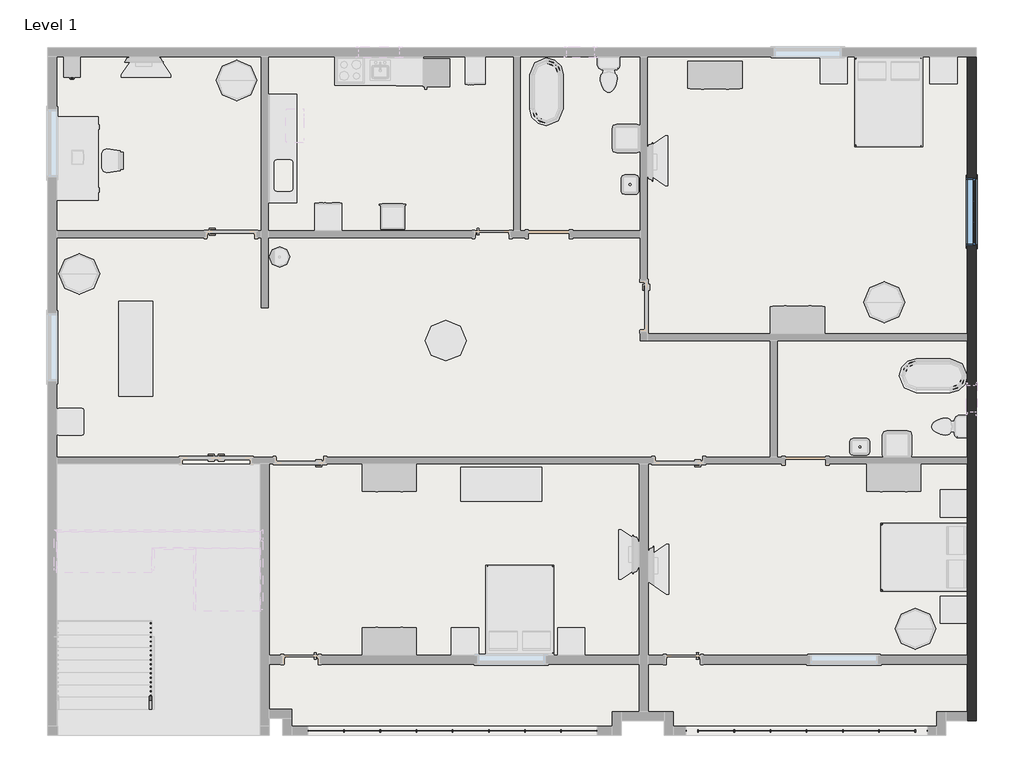
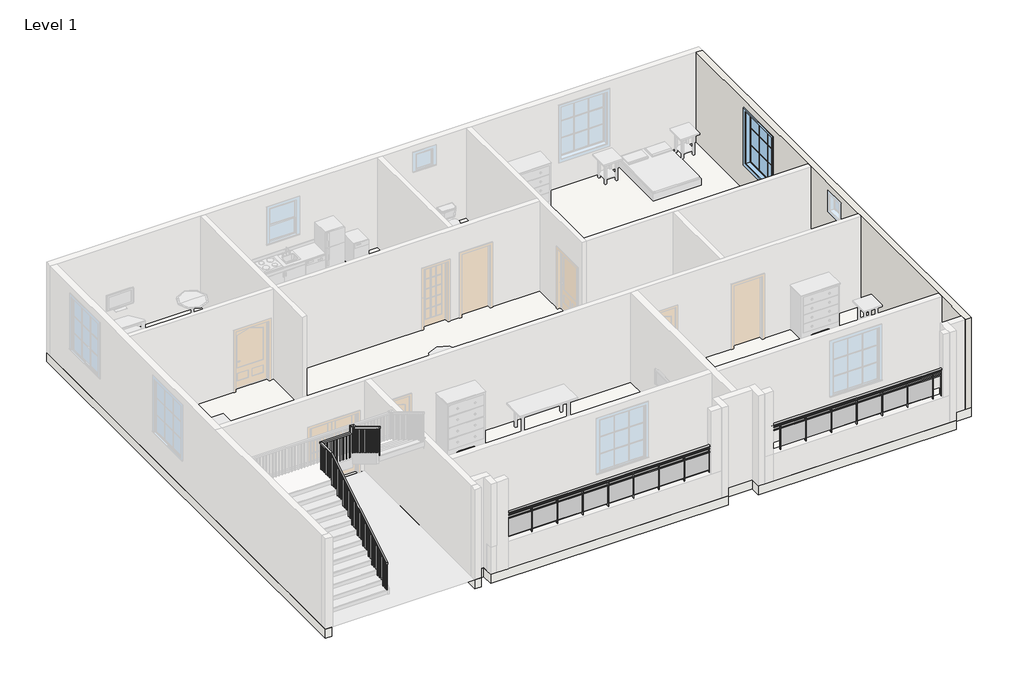
# One storey, part 2 of 4: 3 railings, 1 slab, 1 wall, 1 window.
"""IFC4 building model written with IfcOpenShell, lengths in millimetres."""

from ifc_helpers import new_model, si_unit, point, frame, origin, place, context, project, spatial, polyline, ellipse_curve, trimmed, outline, extrude, faceted_brep, transform, mapped, element, save
from ifc_brep_helpers import plane_surface, extruded_surface, advanced_brep
from components import window_cc15f82e

model = new_model("IFC4")

# Units and contexts
model_context = context("Model", 3, world=origin())
ifc_project = project(units=[si_unit("LENGTHUNIT", "METRE", prefix="MILLI")], contexts=[model_context])

# Site, building, storey
site = spatial("IfcSite", under=ifc_project)
building = spatial("IfcBuilding", under=site)
storey = spatial("IfcBuildingStorey", under=building, Name="Level 1", Elevation=0.0)

# Railings
placement = place(None, origin())
element("IfcRailing", 1, ObjectType="Glass Panel - Bottom Fill", at=placement, inside=storey, context=model_context, shape_type="SolidModel", body=[
    advanced_brep(
    [(-14338.4480019, -638.2741123, 1828.8), (-14338.4480019, -714.4741123, 1828.8), (-7836.0480019, -638.2741123, 1828.8), (-7836.0480019, -714.4741123, 1828.8)],
    [
        (0, 1, ellipse_curve(frame((-14338.4480019, -676.3741123, 1828.8), z_axis=(-1.0, 0.0, 0.0), x_axis=(0.0, -1.0, 0.0)), 38.1, 28.575)),
        (1, 0, ellipse_curve(frame((-14338.4480019, -676.3741123, 1828.8), z_axis=(-1.0, 0.0, 0.0), x_axis=(0.0, -1.0, 0.0)), 38.1, 28.575)),
        (2, 3, ellipse_curve(frame((-7836.0480019, -676.3741123, 1828.8), z_axis=(1.0, 0.0, 0.0), x_axis=(0.0, -1.0, 0.0)), 38.1, 28.575)),
        (3, 2, ellipse_curve(frame((-7836.0480019, -676.3741123, 1828.8), z_axis=(1.0, 0.0, 0.0), x_axis=(0.0, -1.0, 0.0)), 38.1, 28.575)),
        (0, 2),
        (3, 1),
    ],
    [
        plane_surface(frame((-14338.4480019, -676.3741123, 1828.8), z_axis=(-1.0, 0.0, 0.0), x_axis=(0.0, 1.0, 0.0))),
        plane_surface(frame((-7836.0480019, -676.3741123, 1828.8), z_axis=(1.0, 0.0, 0.0), x_axis=(0.0, 1.0, 0.0))),
        extruded_surface(trimmed(ellipse_curve(frame((-7836.0480019, -676.3741123, 1828.8), z_axis=(-1.0, 0.0, 0.0), x_axis=(0.0, -1.0, 0.0)), 38.1, 28.575), [point((-7836.0480019, -638.2741123, 1828.8))], [point((-7836.0480019, -714.4741123, 1828.8))], True, "CARTESIAN"), (-6502.400000000001, 0.0, 0.0), 6502.400000000001),
        extruded_surface(trimmed(ellipse_curve(frame((-7836.0480019, -676.3741123, 1828.8), z_axis=(-1.0, 0.0, 0.0), x_axis=(0.0, -1.0, 0.0)), 38.1, 28.575), [point((-7836.0480019, -714.4741123, 1828.8))], [point((-7836.0480019, -638.2741123, 1828.8))], True, "CARTESIAN"), (-6502.400000000001, 0.0, 0.0), 6502.400000000001),
    ],
    [
        (0, [[1, 2]]),
        (1, [[3, 4]]),
        (2, [[-1, 5, -4, 6]]),
        (3, [[-2, -6, -3, -5]]),
    ],
),
    extrude(outline(polyline([(-14338.4480019, -689.0741123), (-14338.4480019, -663.6741123), (-7836.0480019, -663.6741123), (-7836.0480019, -689.0741123), (-14338.4480019, -689.0741123)])), frame((0.0, 0.0, 1714.5), z_axis=(0.0, 0.0, 1.0), x_axis=(1.0, 0.0, 0.0)), (0.0, 0.0, 1.0), 25.4),
    extrude(outline(polyline([(-14338.4480019, -689.0741123), (-14338.4480019, -663.6741123), (-7836.0480019, -663.6741123), (-7836.0480019, -689.0741123), (-14338.4480019, -689.0741123)])), frame((0.0, 0.0, 1612.9), z_axis=(0.0, 0.0, 1.0), x_axis=(1.0, 0.0, 0.0)), (0.0, 0.0, 1.0), 25.4),
    extrude(outline(polyline([(-8648.8480019, -669.8389552), (-7836.0480019, -669.8389552), (-7836.0480019, -676.1889552), (-8648.8480019, -676.1889552), (-8648.8480019, -669.8389552)])), frame((0.0, 0.0, 1016.0), z_axis=(0.0, 0.0, 1.0), x_axis=(1.0, 0.0, 0.0)), (0.0, 0.0, 1.0), 596.9),
    extrude(outline(polyline([(-8655.1980019, -701.7741123), (-8655.1980019, -650.9741123), (-8642.4980019, -650.9741123), (-8642.4980019, -701.7741123), (-8655.1980019, -701.7741123)])), frame((0.0, 0.0, 914.4), z_axis=(0.0, 0.0, 1.0), x_axis=(1.0, 0.0, 0.0)), (0.0, 0.0, 1.0), 885.6788223),
    extrude(outline(polyline([(-9461.6480019, -669.8389552), (-8648.8480019, -669.8389552), (-8648.8480019, -676.1889552), (-9461.6480019, -676.1889552), (-9461.6480019, -669.8389552)])), frame((0.0, 0.0, 1016.0), z_axis=(0.0, 0.0, 1.0), x_axis=(1.0, 0.0, 0.0)), (0.0, 0.0, 1.0), 596.9),
    extrude(outline(polyline([(-9467.9980019, -701.7741123), (-9467.9980019, -650.9741123), (-9455.2980019, -650.9741123), (-9455.2980019, -701.7741123), (-9467.9980019, -701.7741123)])), frame((0.0, 0.0, 914.4), z_axis=(0.0, 0.0, 1.0), x_axis=(1.0, 0.0, 0.0)), (0.0, 0.0, 1.0), 885.6788223),
    extrude(outline(polyline([(-10274.4480019, -669.8389552), (-9461.6480019, -669.8389552), (-9461.6480019, -676.1889552), (-10274.4480019, -676.1889552), (-10274.4480019, -669.8389552)])), frame((0.0, 0.0, 1016.0), z_axis=(0.0, 0.0, 1.0), x_axis=(1.0, 0.0, 0.0)), (0.0, 0.0, 1.0), 596.9),
    extrude(outline(polyline([(-10280.7980019, -701.7741123), (-10280.7980019, -650.9741123), (-10268.0980019, -650.9741123), (-10268.0980019, -701.7741123), (-10280.7980019, -701.7741123)])), frame((0.0, 0.0, 914.4), z_axis=(0.0, 0.0, 1.0), x_axis=(1.0, 0.0, 0.0)), (0.0, 0.0, 1.0), 885.6788223),
    extrude(outline(polyline([(-11087.2480019, -669.8389552), (-10274.4480019, -669.8389552), (-10274.4480019, -676.1889552), (-11087.2480019, -676.1889552), (-11087.2480019, -669.8389552)])), frame((0.0, 0.0, 1016.0), z_axis=(0.0, 0.0, 1.0), x_axis=(1.0, 0.0, 0.0)), (0.0, 0.0, 1.0), 596.9),
    extrude(outline(polyline([(-11093.5980019, -701.7741123), (-11093.5980019, -650.9741123), (-11080.8980019, -650.9741123), (-11080.8980019, -701.7741123), (-11093.5980019, -701.7741123)])), frame((0.0, 0.0, 914.4), z_axis=(0.0, 0.0, 1.0), x_axis=(1.0, 0.0, 0.0)), (0.0, 0.0, 1.0), 885.6788223),
    extrude(outline(polyline([(-11900.0480019, -669.8389552), (-11087.2480019, -669.8389552), (-11087.2480019, -676.1889552), (-11900.0480019, -676.1889552), (-11900.0480019, -669.8389552)])), frame((0.0, 0.0, 1016.0), z_axis=(0.0, 0.0, 1.0), x_axis=(1.0, 0.0, 0.0)), (0.0, 0.0, 1.0), 596.9),
    extrude(outline(polyline([(-11906.3980019, -701.7741123), (-11906.3980019, -650.9741123), (-11893.6980019, -650.9741123), (-11893.6980019, -701.7741123), (-11906.3980019, -701.7741123)])), frame((0.0, 0.0, 914.4), z_axis=(0.0, 0.0, 1.0), x_axis=(1.0, 0.0, 0.0)), (0.0, 0.0, 1.0), 885.6788223),
    extrude(outline(polyline([(-12712.8480019, -669.8389552), (-11900.0480019, -669.8389552), (-11900.0480019, -676.1889552), (-12712.8480019, -676.1889552), (-12712.8480019, -669.8389552)])), frame((0.0, 0.0, 1016.0), z_axis=(0.0, 0.0, 1.0), x_axis=(1.0, 0.0, 0.0)), (0.0, 0.0, 1.0), 596.9),
    extrude(outline(polyline([(-12719.1980019, -701.7741123), (-12719.1980019, -650.9741123), (-12706.4980019, -650.9741123), (-12706.4980019, -701.7741123), (-12719.1980019, -701.7741123)])), frame((0.0, 0.0, 914.4), z_axis=(0.0, 0.0, 1.0), x_axis=(1.0, 0.0, 0.0)), (0.0, 0.0, 1.0), 885.6788223),
    extrude(outline(polyline([(-13525.6480019, -669.8389552), (-12712.8480019, -669.8389552), (-12712.8480019, -676.1889552), (-13525.6480019, -676.1889552), (-13525.6480019, -669.8389552)])), frame((0.0, 0.0, 1016.0), z_axis=(0.0, 0.0, 1.0), x_axis=(1.0, 0.0, 0.0)), (0.0, 0.0, 1.0), 596.9),
    extrude(outline(polyline([(-13531.9980019, -701.7741123), (-13531.9980019, -650.9741123), (-13519.2980019, -650.9741123), (-13519.2980019, -701.7741123), (-13531.9980019, -701.7741123)])), frame((0.0, 0.0, 914.4), z_axis=(0.0, 0.0, 1.0), x_axis=(1.0, 0.0, 0.0)), (0.0, 0.0, 1.0), 885.6788223),
    extrude(outline(polyline([(-14338.4480019, -669.8389552), (-13525.6480019, -669.8389552), (-13525.6480019, -676.1889552), (-14338.4480019, -676.1889552), (-14338.4480019, -669.8389552)])), frame((0.0, 0.0, 1016.0), z_axis=(0.0, 0.0, 1.0), x_axis=(1.0, 0.0, 0.0)), (0.0, 0.0, 1.0), 596.9),
    extrude(outline(polyline([(-7848.7480019, -685.8991123), (-7848.7480019, -666.8491123), (-7829.6980019, -666.8491123), (-7829.6980019, -685.8991123), (-7848.7480019, -685.8991123)])), frame((0.0, 0.0, 914.4), z_axis=(0.0, 0.0, 1.0), x_axis=(1.0, 0.0, 0.0)), (0.0, 0.0, 1.0), 885.6788223),
    extrude(outline(polyline([(-14344.7980019, -685.8991123), (-14344.7980019, -666.8491123), (-14325.7480019, -666.8491123), (-14325.7480019, -685.8991123), (-14344.7980019, -685.8991123)])), frame((0.0, 0.0, 914.4), z_axis=(0.0, 0.0, 1.0), x_axis=(1.0, 0.0, 0.0)), (0.0, 0.0, 1.0), 885.6788223),
])
element("IfcRailing", 2, ObjectType="Glass Panel - Bottom Fill", at=placement, inside=storey, context=model_context, shape_type="SolidModel", body=[
    advanced_brep(
    [(-5854.8480019, -638.2741123, 1828.8), (-5854.8480019, -714.4741123, 1828.8), (-419.2480019, -638.2741123, 1828.8), (-419.2480019, -714.4741123, 1828.8)],
    [
        (0, 1, ellipse_curve(frame((-5854.8480019, -676.3741123, 1828.8), z_axis=(-1.0, 0.0, 0.0), x_axis=(0.0, -1.0, 0.0)), 38.1, 28.575)),
        (1, 0, ellipse_curve(frame((-5854.8480019, -676.3741123, 1828.8), z_axis=(-1.0, 0.0, 0.0), x_axis=(0.0, -1.0, 0.0)), 38.1, 28.575)),
        (2, 3, ellipse_curve(frame((-419.2480019, -676.3741123, 1828.8), z_axis=(1.0, 0.0, 0.0), x_axis=(0.0, -1.0, 0.0)), 38.1, 28.575)),
        (3, 2, ellipse_curve(frame((-419.2480019, -676.3741123, 1828.8), z_axis=(1.0, 0.0, 0.0), x_axis=(0.0, -1.0, 0.0)), 38.1, 28.575)),
        (0, 2),
        (3, 1),
    ],
    [
        plane_surface(frame((-5854.8480019, -676.3741123, 1828.8), z_axis=(-1.0, 0.0, 0.0), x_axis=(0.0, 1.0, 0.0))),
        plane_surface(frame((-419.2480019, -676.3741123, 1828.8), z_axis=(1.0, 0.0, 0.0), x_axis=(0.0, 1.0, 0.0))),
        extruded_surface(trimmed(ellipse_curve(frame((-419.2480019, -676.3741123, 1828.8), z_axis=(-1.0, 0.0, 0.0), x_axis=(0.0, -1.0, 0.0)), 38.1, 28.575), [point((-419.2480019, -638.2741123, 1828.8))], [point((-419.2480019, -714.4741123, 1828.8))], True, "CARTESIAN"), (-5435.599999999999, 0.0, 0.0), 5435.599999999999),
        extruded_surface(trimmed(ellipse_curve(frame((-419.2480019, -676.3741123, 1828.8), z_axis=(-1.0, 0.0, 0.0), x_axis=(0.0, -1.0, 0.0)), 38.1, 28.575), [point((-419.2480019, -714.4741123, 1828.8))], [point((-419.2480019, -638.2741123, 1828.8))], True, "CARTESIAN"), (-5435.599999999999, 0.0, 0.0), 5435.599999999999),
    ],
    [
        (0, [[1, 2]]),
        (1, [[3, 4]]),
        (2, [[-1, 5, -4, 6]]),
        (3, [[-2, -6, -3, -5]]),
    ],
),
    extrude(outline(polyline([(-5854.8480019, -689.0741123), (-5854.8480019, -663.6741123), (-419.2480019, -663.6741123), (-419.2480019, -689.0741123), (-5854.8480019, -689.0741123)])), frame((0.0, 0.0, 1714.5), z_axis=(0.0, 0.0, 1.0), x_axis=(1.0, 0.0, 0.0)), (0.0, 0.0, 1.0), 25.4),
    extrude(outline(polyline([(-5854.8480019, -689.0741123), (-5854.8480019, -663.6741123), (-419.2480019, -663.6741123), (-419.2480019, -689.0741123), (-5854.8480019, -689.0741123)])), frame((0.0, 0.0, 1612.9), z_axis=(0.0, 0.0, 1.0), x_axis=(1.0, 0.0, 0.0)), (0.0, 0.0, 1.0), 25.4),
    extrude(outline(polyline([(-704.9980019, -701.7741123), (-704.9980019, -650.9741123), (-692.2980019, -650.9741123), (-692.2980019, -701.7741123), (-704.9980019, -701.7741123)])), frame((0.0, 0.0, 914.4), z_axis=(0.0, 0.0, 1.0), x_axis=(1.0, 0.0, 0.0)), (0.0, 0.0, 1.0), 885.6788223),
    extrude(outline(polyline([(-1511.4480019, -669.8389552), (-698.6480019, -669.8389552), (-698.6480019, -676.1889552), (-1511.4480019, -676.1889552), (-1511.4480019, -669.8389552)])), frame((0.0, 0.0, 1016.0), z_axis=(0.0, 0.0, 1.0), x_axis=(1.0, 0.0, 0.0)), (0.0, 0.0, 1.0), 596.9),
    extrude(outline(polyline([(-1517.7980019, -701.7741123), (-1517.7980019, -650.9741123), (-1505.0980019, -650.9741123), (-1505.0980019, -701.7741123), (-1517.7980019, -701.7741123)])), frame((0.0, 0.0, 914.4), z_axis=(0.0, 0.0, 1.0), x_axis=(1.0, 0.0, 0.0)), (0.0, 0.0, 1.0), 885.6788223),
    extrude(outline(polyline([(-2324.2480019, -669.8389552), (-1511.4480019, -669.8389552), (-1511.4480019, -676.1889552), (-2324.2480019, -676.1889552), (-2324.2480019, -669.8389552)])), frame((0.0, 0.0, 1016.0), z_axis=(0.0, 0.0, 1.0), x_axis=(1.0, 0.0, 0.0)), (0.0, 0.0, 1.0), 596.9),
    extrude(outline(polyline([(-2330.5980019, -701.7741123), (-2330.5980019, -650.9741123), (-2317.8980019, -650.9741123), (-2317.8980019, -701.7741123), (-2330.5980019, -701.7741123)])), frame((0.0, 0.0, 914.4), z_axis=(0.0, 0.0, 1.0), x_axis=(1.0, 0.0, 0.0)), (0.0, 0.0, 1.0), 885.6788223),
    extrude(outline(polyline([(-3137.0480019, -669.8389552), (-2324.2480019, -669.8389552), (-2324.2480019, -676.1889552), (-3137.0480019, -676.1889552), (-3137.0480019, -669.8389552)])), frame((0.0, 0.0, 1016.0), z_axis=(0.0, 0.0, 1.0), x_axis=(1.0, 0.0, 0.0)), (0.0, 0.0, 1.0), 596.9),
    extrude(outline(polyline([(-3143.3980019, -701.7741123), (-3143.3980019, -650.9741123), (-3130.6980019, -650.9741123), (-3130.6980019, -701.7741123), (-3143.3980019, -701.7741123)])), frame((0.0, 0.0, 914.4), z_axis=(0.0, 0.0, 1.0), x_axis=(1.0, 0.0, 0.0)), (0.0, 0.0, 1.0), 885.6788223),
    extrude(outline(polyline([(-3949.8480019, -669.8389552), (-3137.0480019, -669.8389552), (-3137.0480019, -676.1889552), (-3949.8480019, -676.1889552), (-3949.8480019, -669.8389552)])), frame((0.0, 0.0, 1016.0), z_axis=(0.0, 0.0, 1.0), x_axis=(1.0, 0.0, 0.0)), (0.0, 0.0, 1.0), 596.9),
    extrude(outline(polyline([(-3956.1980019, -701.7741123), (-3956.1980019, -650.9741123), (-3943.4980019, -650.9741123), (-3943.4980019, -701.7741123), (-3956.1980019, -701.7741123)])), frame((0.0, 0.0, 914.4), z_axis=(0.0, 0.0, 1.0), x_axis=(1.0, 0.0, 0.0)), (0.0, 0.0, 1.0), 885.6788223),
    extrude(outline(polyline([(-4762.6480019, -669.8389552), (-3949.8480019, -669.8389552), (-3949.8480019, -676.1889552), (-4762.6480019, -676.1889552), (-4762.6480019, -669.8389552)])), frame((0.0, 0.0, 1016.0), z_axis=(0.0, 0.0, 1.0), x_axis=(1.0, 0.0, 0.0)), (0.0, 0.0, 1.0), 596.9),
    extrude(outline(polyline([(-4768.9980019, -701.7741123), (-4768.9980019, -650.9741123), (-4756.2980019, -650.9741123), (-4756.2980019, -701.7741123), (-4768.9980019, -701.7741123)])), frame((0.0, 0.0, 914.4), z_axis=(0.0, 0.0, 1.0), x_axis=(1.0, 0.0, 0.0)), (0.0, 0.0, 1.0), 885.6788223),
    extrude(outline(polyline([(-5575.4480019, -669.8389552), (-4762.6480019, -669.8389552), (-4762.6480019, -676.1889552), (-5575.4480019, -676.1889552), (-5575.4480019, -669.8389552)])), frame((0.0, 0.0, 1016.0), z_axis=(0.0, 0.0, 1.0), x_axis=(1.0, 0.0, 0.0)), (0.0, 0.0, 1.0), 596.9),
    extrude(outline(polyline([(-5581.7980019, -701.7741123), (-5581.7980019, -650.9741123), (-5569.0980019, -650.9741123), (-5569.0980019, -701.7741123), (-5581.7980019, -701.7741123)])), frame((0.0, 0.0, 914.4), z_axis=(0.0, 0.0, 1.0), x_axis=(1.0, 0.0, 0.0)), (0.0, 0.0, 1.0), 885.6788223),
    extrude(outline(polyline([(-431.9480019, -685.8991123), (-431.9480019, -666.8491123), (-412.8980019, -666.8491123), (-412.8980019, -685.8991123), (-431.9480019, -685.8991123)])), frame((0.0, 0.0, 914.4), z_axis=(0.0, 0.0, 1.0), x_axis=(1.0, 0.0, 0.0)), (0.0, 0.0, 1.0), 885.6788223),
    extrude(outline(polyline([(-5861.1980019, -685.8991123), (-5861.1980019, -666.8491123), (-5842.1480019, -666.8491123), (-5842.1480019, -685.8991123), (-5861.1980019, -685.8991123)])), frame((0.0, 0.0, 914.4), z_axis=(0.0, 0.0, 1.0), x_axis=(1.0, 0.0, 0.0)), (0.0, 0.0, 1.0), 885.6788223),
])
element("IfcRailing", 3, ObjectType="Handrail - Rectangular", at=placement, inside=storey, context=model_context, shape_type="SolidModel", body=[
    faceted_brep([(-17894.4480019, -193.7741123, 1083.7333333), (-17894.4480019, -193.7741123, 1024.3318731), (-17843.6480019, -193.7741123, 1024.3318731), (-17843.6480019, -193.7741123, 1083.7333333), (-17894.4480019, 2879.6258877, 2946.4), (-17894.4480019, 2893.8182972, 2895.6), (-17843.6480019, 2893.8182972, 2895.6), (-17843.6480019, 2879.6258877, 2946.4), (-17894.4480019, 3489.2258877, 2946.4), (-17894.4480019, 3489.2258877, 2895.6), (-17843.6480019, 3438.4258877, 2895.6), (-17843.6480019, 3438.4258877, 2946.4), (-16802.2480019, 2041.4258877, 3962.4), (-16853.0480019, 2041.4258877, 3962.4), (-16853.0480019, 2041.4258877, 3902.9985397), (-16802.2480019, 2041.4258877, 3902.9985397), (-16802.2480019, 3348.0334783, 3111.1151515), (-16802.2480019, 3362.2258877, 3161.9151515), (-16853.0480019, 3348.0334783, 3111.1151515), (-16853.0480019, 3362.2258877, 3161.9151515), (-16929.2480019, 3489.2258877, 2946.4), (-16878.4480019, 3489.2258877, 2895.6), (-16878.4480019, 3438.4258877, 2895.6), (-16929.2480019, 3438.4258877, 2946.4), (-16929.2480019, 3489.2258877, 3161.9151515), (-16878.4480019, 3489.2258877, 3111.1151515), (-16878.4480019, 3438.4258877, 3111.1151515), (-16929.2480019, 3438.4258877, 3161.9151515), (-16802.2480019, 3489.2258877, 3161.9151515), (-16802.2480019, 3489.2258877, 3111.1151515), (-16853.0480019, 3438.4258877, 3111.1151515), (-16853.0480019, 3438.4258877, 3161.9151515)], [[[0, 1, 2, 3]], [[1, 0, 4, 5]], [[2, 1, 5, 6]], [[3, 2, 6, 7]], [[0, 3, 7, 4]], [[5, 4, 8, 9]], [[6, 5, 9, 10]], [[7, 6, 10, 11]], [[4, 7, 11, 8]], [[12, 13, 14, 15]], [[16, 17, 12, 15]], [[18, 16, 15, 14]], [[19, 18, 14, 13]], [[17, 19, 13, 12]], [[9, 8, 20, 21]], [[10, 9, 21, 22]], [[11, 10, 22, 23]], [[8, 11, 23, 20]], [[21, 20, 24, 25]], [[22, 21, 25, 26]], [[23, 22, 26, 27]], [[20, 23, 27, 24]], [[25, 24, 28, 29]], [[26, 25, 29, 30]], [[27, 26, 30, 31]], [[24, 27, 31, 28]], [[29, 28, 17, 16]], [[30, 29, 16, 18]], [[31, 30, 18, 19]], [[28, 31, 19, 17]]]),
    extrude(outline(polyline([(2133.5008877, 3847.1955094), (2152.5508877, 3835.6500549), (2152.5508877, 2878.6666667), (2133.5008877, 2878.6666667), (2133.5008877, 3847.1955094)])), frame((-16837.1730019, 0.0, 0.0), z_axis=(1.0, 0.0, 0.0), x_axis=(0.0, 1.0, 0.0)), (0.0, 0.0, 1.0), 19.05),
    extrude(outline(polyline([(2235.1008877, 3785.6197519), (2254.1508877, 3774.0742973), (2254.1508877, 2878.6666667), (2235.1008877, 2878.6666667), (2235.1008877, 3785.6197519)])), frame((-16837.1730019, 0.0, 0.0), z_axis=(1.0, 0.0, 0.0), x_axis=(0.0, 1.0, 0.0)), (0.0, 0.0, 1.0), 19.05),
    extrude(outline(polyline([(2336.7008877, 3724.0439943), (2355.7508877, 3712.4985397), (2355.7508877, 2709.3333333), (2336.7008877, 2709.3333333), (2336.7008877, 3724.0439943)])), frame((-16837.1730019, 0.0, 0.0), z_axis=(1.0, 0.0, 0.0), x_axis=(0.0, 1.0, 0.0)), (0.0, 0.0, 1.0), 19.05),
    extrude(outline(polyline([(2438.3008877, 3662.4682367), (2457.3508877, 3650.9227822), (2457.3508877, 2709.3333333), (2438.3008877, 2709.3333333), (2438.3008877, 3662.4682367)])), frame((-16837.1730019, 0.0, 0.0), z_axis=(1.0, 0.0, 0.0), x_axis=(0.0, 1.0, 0.0)), (0.0, 0.0, 1.0), 19.05),
    extrude(outline(polyline([(2539.9008877, 3600.8924791), (2558.9508877, 3589.3470246), (2558.9508877, 2709.3333333), (2539.9008877, 2709.3333333), (2539.9008877, 3600.8924791)])), frame((-16837.1730019, 0.0, 0.0), z_axis=(1.0, 0.0, 0.0), x_axis=(0.0, 1.0, 0.0)), (0.0, 0.0, 1.0), 19.05),
    extrude(outline(polyline([(2641.5008877, 3539.3167216), (2660.5508877, 3527.771267), (2660.5508877, 2540.0), (2641.5008877, 2540.0), (2641.5008877, 3539.3167216)])), frame((-16837.1730019, 0.0, 0.0), z_axis=(1.0, 0.0, 0.0), x_axis=(0.0, 1.0, 0.0)), (0.0, 0.0, 1.0), 19.05),
    extrude(outline(polyline([(2743.1008877, 3477.740964), (2762.1508877, 3466.1955094), (2762.1508877, 2540.0), (2743.1008877, 2540.0), (2743.1008877, 3477.740964)])), frame((-16837.1730019, 0.0, 0.0), z_axis=(1.0, 0.0, 0.0), x_axis=(0.0, 1.0, 0.0)), (0.0, 0.0, 1.0), 19.05),
    extrude(outline(polyline([(2844.7008877, 3416.1652064), (2863.7508877, 3404.6197519), (2863.7508877, 2540.0), (2844.7008877, 2540.0), (2844.7008877, 3416.1652064)])), frame((-16837.1730019, 0.0, 0.0), z_axis=(1.0, 0.0, 0.0), x_axis=(0.0, 1.0, 0.0)), (0.0, 0.0, 1.0), 19.05),
    extrude(outline(polyline([(2946.3008877, 3354.5894488), (2965.3508877, 3343.0439943), (2965.3508877, 2370.6666667), (2946.3008877, 2370.6666667), (2946.3008877, 3354.5894488)])), frame((-16837.1730019, 0.0, 0.0), z_axis=(1.0, 0.0, 0.0), x_axis=(0.0, 1.0, 0.0)), (0.0, 0.0, 1.0), 19.05),
    extrude(outline(polyline([(3047.9008877, 3293.0136913), (3066.9508877, 3281.4682367), (3066.9508877, 2370.6666667), (3047.9008877, 2370.6666667), (3047.9008877, 3293.0136913)])), frame((-16837.1730019, 0.0, 0.0), z_axis=(1.0, 0.0, 0.0), x_axis=(0.0, 1.0, 0.0)), (0.0, 0.0, 1.0), 19.05),
    extrude(outline(polyline([(3149.5008877, 3231.4379337), (3168.5508877, 3219.8924791), (3168.5508877, 2370.6666667), (3149.5008877, 2370.6666667), (3149.5008877, 3231.4379337)])), frame((-16837.1730019, 0.0, 0.0), z_axis=(1.0, 0.0, 0.0), x_axis=(0.0, 1.0, 0.0)), (0.0, 0.0, 1.0), 19.05),
    extrude(outline(polyline([(3251.1008877, 3169.8621761), (3270.1508877, 3158.3167216), (3270.1508877, 2201.3333333), (3251.1008877, 2201.3333333), (3251.1008877, 3169.8621761)])), frame((-16837.1730019, 0.0, 0.0), z_axis=(1.0, 0.0, 0.0), x_axis=(0.0, 1.0, 0.0)), (0.0, 0.0, 1.0), 19.05),
    extrude(outline(polyline([(-16837.1730019, 3371.7508877), (-16818.1230019, 3371.7508877), (-16818.1230019, 3352.7008877), (-16837.1730019, 3352.7008877), (-16837.1730019, 3371.7508877)])), frame((0.0, 0.0, 2201.3333333), z_axis=(0.0, 0.0, 1.0), x_axis=(1.0, 0.0, 0.0)), (0.0, 0.0, 1.0), 909.7818182),
    extrude(outline(polyline([(-16862.5730019, 3454.3008877), (-16862.5730019, 3473.3508877), (-16843.5230019, 3473.3508877), (-16843.5230019, 3454.3008877), (-16862.5730019, 3454.3008877)])), frame((0.0, 0.0, 2032.0), z_axis=(0.0, 0.0, 1.0), x_axis=(1.0, 0.0, 0.0)), (0.0, 0.0, 1.0), 1079.1151515),
    extrude(outline(polyline([(-16964.1730019, 3454.3008877), (-16964.1730019, 3473.3508877), (-16945.1230019, 3473.3508877), (-16945.1230019, 3454.3008877), (-16964.1730019, 3454.3008877)])), frame((0.0, 0.0, 2032.0), z_axis=(0.0, 0.0, 1.0), x_axis=(1.0, 0.0, 0.0)), (0.0, 0.0, 1.0), 863.6),
    extrude(outline(polyline([(-17065.7730019, 3454.3008877), (-17065.7730019, 3473.3508877), (-17046.7230019, 3473.3508877), (-17046.7230019, 3454.3008877), (-17065.7730019, 3454.3008877)])), frame((0.0, 0.0, 2032.0), z_axis=(0.0, 0.0, 1.0), x_axis=(1.0, 0.0, 0.0)), (0.0, 0.0, 1.0), 863.6),
    extrude(outline(polyline([(-17167.3730019, 3454.3008877), (-17167.3730019, 3473.3508877), (-17148.3230019, 3473.3508877), (-17148.3230019, 3454.3008877), (-17167.3730019, 3454.3008877)])), frame((0.0, 0.0, 2032.0), z_axis=(0.0, 0.0, 1.0), x_axis=(1.0, 0.0, 0.0)), (0.0, 0.0, 1.0), 863.6),
    extrude(outline(polyline([(-17268.9730019, 3454.3008877), (-17268.9730019, 3473.3508877), (-17249.9230019, 3473.3508877), (-17249.9230019, 3454.3008877), (-17268.9730019, 3454.3008877)])), frame((0.0, 0.0, 2032.0), z_axis=(0.0, 0.0, 1.0), x_axis=(1.0, 0.0, 0.0)), (0.0, 0.0, 1.0), 863.6),
    extrude(outline(polyline([(-17370.5730019, 3454.3008877), (-17370.5730019, 3473.3508877), (-17351.5230019, 3473.3508877), (-17351.5230019, 3454.3008877), (-17370.5730019, 3454.3008877)])), frame((0.0, 0.0, 2032.0), z_axis=(0.0, 0.0, 1.0), x_axis=(1.0, 0.0, 0.0)), (0.0, 0.0, 1.0), 863.6),
    extrude(outline(polyline([(-17472.1730019, 3454.3008877), (-17472.1730019, 3473.3508877), (-17453.1230019, 3473.3508877), (-17453.1230019, 3454.3008877), (-17472.1730019, 3454.3008877)])), frame((0.0, 0.0, 2032.0), z_axis=(0.0, 0.0, 1.0), x_axis=(1.0, 0.0, 0.0)), (0.0, 0.0, 1.0), 863.6),
    extrude(outline(polyline([(-17573.7730019, 3454.3008877), (-17573.7730019, 3473.3508877), (-17554.7230019, 3473.3508877), (-17554.7230019, 3454.3008877), (-17573.7730019, 3454.3008877)])), frame((0.0, 0.0, 2032.0), z_axis=(0.0, 0.0, 1.0), x_axis=(1.0, 0.0, 0.0)), (0.0, 0.0, 1.0), 863.6),
    extrude(outline(polyline([(-17675.3730019, 3454.3008877), (-17675.3730019, 3473.3508877), (-17656.3230019, 3473.3508877), (-17656.3230019, 3454.3008877), (-17675.3730019, 3454.3008877)])), frame((0.0, 0.0, 2032.0), z_axis=(0.0, 0.0, 1.0), x_axis=(1.0, 0.0, 0.0)), (0.0, 0.0, 1.0), 863.6),
    extrude(outline(polyline([(-17776.9730019, 3454.3008877), (-17776.9730019, 3473.3508877), (-17757.9230019, 3473.3508877), (-17757.9230019, 3454.3008877), (-17776.9730019, 3454.3008877)])), frame((0.0, 0.0, 2032.0), z_axis=(0.0, 0.0, 1.0), x_axis=(1.0, 0.0, 0.0)), (0.0, 0.0, 1.0), 863.6),
    extrude(outline(polyline([(-17859.5230019, 3378.1008877), (-17878.5730019, 3378.1008877), (-17878.5730019, 3397.1508877), (-17859.5230019, 3397.1508877), (-17859.5230019, 3378.1008877)])), frame((0.0, 0.0, 2032.0), z_axis=(0.0, 0.0, 1.0), x_axis=(1.0, 0.0, 0.0)), (0.0, 0.0, 1.0), 863.6),
    extrude(outline(polyline([(-17859.5230019, 3276.5008877), (-17878.5730019, 3276.5008877), (-17878.5730019, 3295.5508877), (-17859.5230019, 3295.5508877), (-17859.5230019, 3276.5008877)])), frame((0.0, 0.0, 2032.0), z_axis=(0.0, 0.0, 1.0), x_axis=(1.0, 0.0, 0.0)), (0.0, 0.0, 1.0), 863.6),
    extrude(outline(polyline([(-17859.5230019, 3174.9008877), (-17878.5730019, 3174.9008877), (-17878.5730019, 3193.9508877), (-17859.5230019, 3193.9508877), (-17859.5230019, 3174.9008877)])), frame((0.0, 0.0, 2032.0), z_axis=(0.0, 0.0, 1.0), x_axis=(1.0, 0.0, 0.0)), (0.0, 0.0, 1.0), 863.6),
    extrude(outline(polyline([(-17859.5230019, 3073.3008877), (-17878.5730019, 3073.3008877), (-17878.5730019, 3092.3508877), (-17859.5230019, 3092.3508877), (-17859.5230019, 3073.3008877)])), frame((0.0, 0.0, 2032.0), z_axis=(0.0, 0.0, 1.0), x_axis=(1.0, 0.0, 0.0)), (0.0, 0.0, 1.0), 863.6),
    extrude(outline(polyline([(-17859.5230019, 2971.7008877), (-17878.5730019, 2971.7008877), (-17878.5730019, 2990.7508877), (-17859.5230019, 2990.7508877), (-17859.5230019, 2971.7008877)])), frame((0.0, 0.0, 2032.0), z_axis=(0.0, 0.0, 1.0), x_axis=(1.0, 0.0, 0.0)), (0.0, 0.0, 1.0), 863.6),
    extrude(outline(polyline([(2844.7008877, 2865.8318731), (2863.7508877, 2877.3773276), (2863.7508877, 1862.6666667), (2844.7008877, 1862.6666667), (2844.7008877, 2865.8318731)])), frame((-17878.5730019, 0.0, 0.0), z_axis=(1.0, 0.0, 0.0), x_axis=(0.0, 1.0, 0.0)), (0.0, 0.0, 1.0), 19.05),
    extrude(outline(polyline([(2743.1008877, 2804.2561155), (2762.1508877, 2815.80157), (2762.1508877, 1862.6666667), (2743.1008877, 1862.6666667), (2743.1008877, 2804.2561155)])), frame((-17878.5730019, 0.0, 0.0), z_axis=(1.0, 0.0, 0.0), x_axis=(0.0, 1.0, 0.0)), (0.0, 0.0, 1.0), 19.05),
    extrude(outline(polyline([(2641.5008877, 2742.6803579), (2660.5508877, 2754.2258125), (2660.5508877, 1862.6666667), (2641.5008877, 1862.6666667), (2641.5008877, 2742.6803579)])), frame((-17878.5730019, 0.0, 0.0), z_axis=(1.0, 0.0, 0.0), x_axis=(0.0, 1.0, 0.0)), (0.0, 0.0, 1.0), 19.05),
    extrude(outline(polyline([(2539.9008877, 2681.1046004), (2558.9508877, 2692.6500549), (2558.9508877, 1693.3333333), (2539.9008877, 1693.3333333), (2539.9008877, 2681.1046004)])), frame((-17878.5730019, 0.0, 0.0), z_axis=(1.0, 0.0, 0.0), x_axis=(0.0, 1.0, 0.0)), (0.0, 0.0, 1.0), 19.05),
    extrude(outline(polyline([(2438.3008877, 2619.5288428), (2457.3508877, 2631.0742973), (2457.3508877, 1693.3333333), (2438.3008877, 1693.3333333), (2438.3008877, 2619.5288428)])), frame((-17878.5730019, 0.0, 0.0), z_axis=(1.0, 0.0, 0.0), x_axis=(0.0, 1.0, 0.0)), (0.0, 0.0, 1.0), 19.05),
    extrude(outline(polyline([(2336.7008877, 2557.9530852), (2355.7508877, 2569.4985397), (2355.7508877, 1693.3333333), (2336.7008877, 1693.3333333), (2336.7008877, 2557.9530852)])), frame((-17878.5730019, 0.0, 0.0), z_axis=(1.0, 0.0, 0.0), x_axis=(0.0, 1.0, 0.0)), (0.0, 0.0, 1.0), 19.05),
    extrude(outline(polyline([(2235.1008877, 2496.3773276), (2254.1508877, 2507.9227822), (2254.1508877, 1524.0), (2235.1008877, 1524.0), (2235.1008877, 2496.3773276)])), frame((-17878.5730019, 0.0, 0.0), z_axis=(1.0, 0.0, 0.0), x_axis=(0.0, 1.0, 0.0)), (0.0, 0.0, 1.0), 19.05),
    extrude(outline(polyline([(2133.5008877, 2434.80157), (2152.5508877, 2446.3470246), (2152.5508877, 1524.0), (2133.5008877, 1524.0), (2133.5008877, 2434.80157)])), frame((-17878.5730019, 0.0, 0.0), z_axis=(1.0, 0.0, 0.0), x_axis=(0.0, 1.0, 0.0)), (0.0, 0.0, 1.0), 19.05),
    extrude(outline(polyline([(2031.9008877, 2373.2258125), (2050.9508877, 2384.771267), (2050.9508877, 1524.0), (2031.9008877, 1524.0), (2031.9008877, 2373.2258125)])), frame((-17878.5730019, 0.0, 0.0), z_axis=(1.0, 0.0, 0.0), x_axis=(0.0, 1.0, 0.0)), (0.0, 0.0, 1.0), 19.05),
    extrude(outline(polyline([(1930.3008877, 2311.6500549), (1949.3508877, 2323.1955094), (1949.3508877, 1354.6666667), (1930.3008877, 1354.6666667), (1930.3008877, 2311.6500549)])), frame((-17878.5730019, 0.0, 0.0), z_axis=(1.0, 0.0, 0.0), x_axis=(0.0, 1.0, 0.0)), (0.0, 0.0, 1.0), 19.05),
    extrude(outline(polyline([(1828.7008877, 2250.0742973), (1847.7508877, 2261.6197519), (1847.7508877, 1354.6666667), (1828.7008877, 1354.6666667), (1828.7008877, 2250.0742973)])), frame((-17878.5730019, 0.0, 0.0), z_axis=(1.0, 0.0, 0.0), x_axis=(0.0, 1.0, 0.0)), (0.0, 0.0, 1.0), 19.05),
    extrude(outline(polyline([(1727.1008877, 2188.4985397), (1746.1508877, 2200.0439943), (1746.1508877, 1185.3333333), (1727.1008877, 1185.3333333), (1727.1008877, 2188.4985397)])), frame((-17878.5730019, 0.0, 0.0), z_axis=(1.0, 0.0, 0.0), x_axis=(0.0, 1.0, 0.0)), (0.0, 0.0, 1.0), 19.05),
    extrude(outline(polyline([(1625.5008877, 2126.9227822), (1644.5508877, 2138.4682367), (1644.5508877, 1185.3333333), (1625.5008877, 1185.3333333), (1625.5008877, 2126.9227822)])), frame((-17878.5730019, 0.0, 0.0), z_axis=(1.0, 0.0, 0.0), x_axis=(0.0, 1.0, 0.0)), (0.0, 0.0, 1.0), 19.05),
    extrude(outline(polyline([(1523.9008877, 2065.3470246), (1542.9508877, 2076.8924791), (1542.9508877, 1185.3333333), (1523.9008877, 1185.3333333), (1523.9008877, 2065.3470246)])), frame((-17878.5730019, 0.0, 0.0), z_axis=(1.0, 0.0, 0.0), x_axis=(0.0, 1.0, 0.0)), (0.0, 0.0, 1.0), 19.05),
    extrude(outline(polyline([(1422.3008877, 2003.771267), (1441.3508877, 2015.3167216), (1441.3508877, 1016.0), (1422.3008877, 1016.0), (1422.3008877, 2003.771267)])), frame((-17878.5730019, 0.0, 0.0), z_axis=(1.0, 0.0, 0.0), x_axis=(0.0, 1.0, 0.0)), (0.0, 0.0, 1.0), 19.05),
    extrude(outline(polyline([(1320.7008877, 1942.1955094), (1339.7508877, 1953.740964), (1339.7508877, 1016.0), (1320.7008877, 1016.0), (1320.7008877, 1942.1955094)])), frame((-17878.5730019, 0.0, 0.0), z_axis=(1.0, 0.0, 0.0), x_axis=(0.0, 1.0, 0.0)), (0.0, 0.0, 1.0), 19.05),
    extrude(outline(polyline([(1219.1008877, 1880.6197519), (1238.1508877, 1892.1652064), (1238.1508877, 1016.0), (1219.1008877, 1016.0), (1219.1008877, 1880.6197519)])), frame((-17878.5730019, 0.0, 0.0), z_axis=(1.0, 0.0, 0.0), x_axis=(0.0, 1.0, 0.0)), (0.0, 0.0, 1.0), 19.05),
    extrude(outline(polyline([(1117.5008877, 1819.0439943), (1136.5508877, 1830.5894488), (1136.5508877, 846.6666667), (1117.5008877, 846.6666667), (1117.5008877, 1819.0439943)])), frame((-17878.5730019, 0.0, 0.0), z_axis=(1.0, 0.0, 0.0), x_axis=(0.0, 1.0, 0.0)), (0.0, 0.0, 1.0), 19.05),
    extrude(outline(polyline([(1015.9008877, 1757.4682367), (1034.9508877, 1769.0136913), (1034.9508877, 846.6666667), (1015.9008877, 846.6666667), (1015.9008877, 1757.4682367)])), frame((-17878.5730019, 0.0, 0.0), z_axis=(1.0, 0.0, 0.0), x_axis=(0.0, 1.0, 0.0)), (0.0, 0.0, 1.0), 19.05),
    extrude(outline(polyline([(914.3008877, 1695.8924791), (933.3508877, 1707.4379337), (933.3508877, 846.6666667), (914.3008877, 846.6666667), (914.3008877, 1695.8924791)])), frame((-17878.5730019, 0.0, 0.0), z_axis=(1.0, 0.0, 0.0), x_axis=(0.0, 1.0, 0.0)), (0.0, 0.0, 1.0), 19.05),
    extrude(outline(polyline([(812.7008877, 1634.3167216), (831.7508877, 1645.8621761), (831.7508877, 677.3333333), (812.7008877, 677.3333333), (812.7008877, 1634.3167216)])), frame((-17878.5730019, 0.0, 0.0), z_axis=(1.0, 0.0, 0.0), x_axis=(0.0, 1.0, 0.0)), (0.0, 0.0, 1.0), 19.05),
    extrude(outline(polyline([(711.1008877, 1572.740964), (730.1508877, 1584.2864185), (730.1508877, 677.3333333), (711.1008877, 677.3333333), (711.1008877, 1572.740964)])), frame((-17878.5730019, 0.0, 0.0), z_axis=(1.0, 0.0, 0.0), x_axis=(0.0, 1.0, 0.0)), (0.0, 0.0, 1.0), 19.05),
    extrude(outline(polyline([(609.5008877, 1511.1652064), (628.5508877, 1522.710661), (628.5508877, 508.0), (609.5008877, 508.0), (609.5008877, 1511.1652064)])), frame((-17878.5730019, 0.0, 0.0), z_axis=(1.0, 0.0, 0.0), x_axis=(0.0, 1.0, 0.0)), (0.0, 0.0, 1.0), 19.05),
    extrude(outline(polyline([(507.9008877, 1449.5894488), (526.9508877, 1461.1349034), (526.9508877, 508.0), (507.9008877, 508.0), (507.9008877, 1449.5894488)])), frame((-17878.5730019, 0.0, 0.0), z_axis=(1.0, 0.0, 0.0), x_axis=(0.0, 1.0, 0.0)), (0.0, 0.0, 1.0), 19.05),
    extrude(outline(polyline([(406.3008877, 1388.0136913), (425.3508877, 1399.5591458), (425.3508877, 508.0), (406.3008877, 508.0), (406.3008877, 1388.0136913)])), frame((-17878.5730019, 0.0, 0.0), z_axis=(1.0, 0.0, 0.0), x_axis=(0.0, 1.0, 0.0)), (0.0, 0.0, 1.0), 19.05),
    extrude(outline(polyline([(304.7008877, 1326.4379337), (323.7508877, 1337.9833882), (323.7508877, 338.6666667), (304.7008877, 338.6666667), (304.7008877, 1326.4379337)])), frame((-17878.5730019, 0.0, 0.0), z_axis=(1.0, 0.0, 0.0), x_axis=(0.0, 1.0, 0.0)), (0.0, 0.0, 1.0), 19.05),
    extrude(outline(polyline([(203.1008877, 1264.8621761), (222.1508877, 1276.4076307), (222.1508877, 338.6666667), (203.1008877, 338.6666667), (203.1008877, 1264.8621761)])), frame((-17878.5730019, 0.0, 0.0), z_axis=(1.0, 0.0, 0.0), x_axis=(0.0, 1.0, 0.0)), (0.0, 0.0, 1.0), 19.05),
    extrude(outline(polyline([(101.5008877, 1203.2864185), (120.5508877, 1214.8318731), (120.5508877, 338.6666667), (101.5008877, 338.6666667), (101.5008877, 1203.2864185)])), frame((-17878.5730019, 0.0, 0.0), z_axis=(1.0, 0.0, 0.0), x_axis=(0.0, 1.0, 0.0)), (0.0, 0.0, 1.0), 19.05),
    extrude(outline(polyline([(-0.0991123, 1141.710661), (18.9508877, 1153.2561155), (18.9508877, 169.3333333), (-0.0991123, 169.3333333), (-0.0991123, 1141.710661)])), frame((-17878.5730019, 0.0, 0.0), z_axis=(1.0, 0.0, 0.0), x_axis=(0.0, 1.0, 0.0)), (0.0, 0.0, 1.0), 19.05),
    extrude(outline(polyline([(-101.6991123, 1080.1349034), (-82.6491123, 1091.6803579), (-82.6491123, 169.3333333), (-101.6991123, 169.3333333), (-101.6991123, 1080.1349034)])), frame((-17878.5730019, 0.0, 0.0), z_axis=(1.0, 0.0, 0.0), x_axis=(0.0, 1.0, 0.0)), (0.0, 0.0, 1.0), 19.05),
    extrude(outline(polyline([(-16837.1730019, 3473.3508877), (-16818.1230019, 3473.3508877), (-16818.1230019, 3454.3008877), (-16837.1730019, 3454.3008877), (-16837.1730019, 3473.3508877)])), frame((0.0, 0.0, 2032.0), z_axis=(0.0, 0.0, 1.0), x_axis=(1.0, 0.0, 0.0)), (0.0, 0.0, 1.0), 1079.1151515),
    extrude(outline(polyline([(-17859.5230019, 3454.3008877), (-17878.5730019, 3454.3008877), (-17878.5730019, 3473.3508877), (-17859.5230019, 3473.3508877), (-17859.5230019, 3454.3008877)])), frame((0.0, 0.0, 2032.0), z_axis=(0.0, 0.0, 1.0), x_axis=(1.0, 0.0, 0.0)), (0.0, 0.0, 1.0), 863.6),
    extrude(outline(polyline([(-17859.5230019, 2870.1008877), (-17878.5730019, 2870.1008877), (-17878.5730019, 2889.1508877), (-17859.5230019, 2889.1508877), (-17859.5230019, 2870.1008877)])), frame((0.0, 0.0, 2032.0), z_axis=(0.0, 0.0, 1.0), x_axis=(1.0, 0.0, 0.0)), (0.0, 0.0, 1.0), 863.6),
    extrude(outline(polyline([(2041.4258877, 3902.9985397), (2060.4758877, 3891.4530852), (2060.4758877, 2878.6666667), (2041.4258877, 2878.6666667), (2041.4258877, 3902.9985397)])), frame((-16837.1730019, 0.0, 0.0), z_axis=(1.0, 0.0, 0.0), x_axis=(0.0, 1.0, 0.0)), (0.0, 0.0, 1.0), 19.05),
    extrude(outline(polyline([(-193.7741123, 1024.3318731), (-174.7241123, 1035.8773276), (-174.7241123, 169.3333333), (-193.7741123, 169.3333333), (-193.7741123, 1024.3318731)])), frame((-17878.5730019, 0.0, 0.0), z_axis=(1.0, 0.0, 0.0), x_axis=(0.0, 1.0, 0.0)), (0.0, 0.0, 1.0), 19.05),
])

# Slab
element("IfcSlab", 4, ObjectType="Generic - 12\"", at=placement, inside=storey, context=model_context, shape_type="SweptSolid", body=[
    extrude(outline(polyline([(672.9519981, 14665.2258877), (672.9519981, -447.7741123), (-12.8480019, -447.7741123), (-12.8480019, -777.9741123), (-6337.4480019, -777.9741123), (-6337.4480019, -447.7741123), (-7302.6480019, -447.7741123), (-7302.6480019, -777.9741123), (-14897.2480019, -777.9741123), (-14897.2480019, -396.9741123), (-15202.0480019, -396.9741123), (-15202.0480019, -777.9741123), (-15405.2480019, -777.9741123), (-15405.2480019, 5318.0258877), (-19977.2480019, 5318.0258877), (-19977.2480019, -777.9741123), (-20180.4480019, -777.9741123), (-20180.4480019, 14665.2258877), (672.9519981, 14665.2258877)])), frame((0.0, 0.0, -304.8), z_axis=(0.0, 0.0, 1.0), x_axis=(1.0, 0.0, 0.0)), (0.0, 0.0, 1.0), 304.8),
])

# Wall
element("IfcWall", 5, ObjectType="Generic - 8\"", at=placement, inside=storey, context=model_context, shape_type="Brep", body=[
    faceted_brep([(469.7519981, 14462.0258877, 0.0), (469.7519981, 8239.0258877, 0.0), (469.7519981, 8086.6258877, 0.0), (469.7519981, 5470.4258877, 0.0), (469.7519981, 5318.0258877, 0.0), (469.7519981, 1025.4258877, 0.0), (469.7519981, 822.2258877, 0.0), (469.7519981, -244.5741123, 0.0), (469.7519981, -447.7741123, 0.0), (469.7519981, -447.7741123, 3048.0), (469.7519981, -244.5741123, 3048.0), (469.7519981, 822.2258877, 3048.0), (469.7519981, 1025.4258877, 3048.0), (469.7519981, 5318.0258877, 3048.0), (469.7519981, 5470.4258877, 3048.0), (469.7519981, 8086.6258877, 3048.0), (469.7519981, 8239.0258877, 3048.0), (469.7519981, 14462.0258877, 3048.0), (469.7519981, 10220.2258877, 2743.2), (469.7519981, 10220.2258877, 914.4), (469.7519981, 11744.2258877, 914.4), (469.7519981, 11744.2258877, 2743.2), (469.7519981, 6473.7258877, 2768.6), (469.7519981, 6473.7258877, 2159.0), (469.7519981, 7083.3258877, 2159.0), (469.7519981, 7083.3258877, 2768.6), (672.9519981, 14462.0258877, 0.0), (672.9519981, 14462.0258877, 3048.0), (672.9519981, -447.7741123, 3048.0), (672.9519981, -447.7741123, 0.0), (672.9519981, 10220.2258877, 2743.2), (672.9519981, 11744.2258877, 2743.2), (672.9519981, 11744.2258877, 914.4), (672.9519981, 10220.2258877, 914.4), (672.9519981, 6473.7258877, 2768.6), (672.9519981, 7083.3258877, 2768.6), (672.9519981, 7083.3258877, 2159.0), (672.9519981, 6473.7258877, 2159.0)], [[[0, 1, 2, 3, 4, 5, 6, 7, 8, 9, 10, 11, 12, 13, 14, 15, 16, 17], [18, 19, 20, 21], [22, 23, 24, 25]], [[26, 27, 28, 29], [30, 31, 32, 33], [34, 35, 36, 37]], [[8, 7, 6, 5, 4, 3, 2, 1, 0, 26, 29]], [[9, 8, 29, 28]], [[0, 17, 27, 26]], [[19, 18, 30, 33]], [[20, 19, 33, 32]], [[21, 20, 32, 31]], [[18, 21, 31, 30]], [[23, 22, 34, 37]], [[24, 23, 37, 36]], [[25, 24, 36, 35]], [[22, 25, 35, 34]], [[17, 16, 15, 14, 13, 12, 11, 10, 9, 28, 27]]]),
])

# Window
window_shape = window_cc15f82e(model_context)
element("IfcWindow", 6, ObjectType="Casement 3x3 with Trim : 60\" x 72\"", at=placement, inside=storey, context=model_context, shape_type="MappedRepresentation", body=[
    mapped(window_shape, transform((571.3519981, 10982.2258877, 609.6), x_axis=(0.0, -1.0, 0.0), y_axis=(1.0, 0.0, 0.0), z_axis=(0.0, 0.0, 1.0))),
])

save(model, "model.ifc")

# Revit data of these elements
# Type "Glass Panel - Bottom Fill"
#   Assembly Code = "C2010400"
#   built-in parameter 1008612 = 0.0416667 (stored number, unit not read)
#   built-in parameter 1008611 = 0.0416667 (stored number, unit not read)
#   built-in parameter 1008609 = 0.333333 (stored number, unit not read)
#   built-in parameter 1008604 = 0.166667 (stored number, unit not read)
#   built-in parameter 1008603 = 0.166667 (stored number, unit not read)
#   Railing Height = 3' - 0"
#   built-in parameter 1008630 = 2
#   built-in parameter 1008610 = 2
#   built-in parameter 1008618 = Baluster - Square : 3/4"
# Type "Handrail - Rectangular"
#   Assembly Code = "C2010400"
#   built-in parameter 1008612 = 0.0416667 (stored number, unit not read)
#   built-in parameter 1008611 = 0.0416667 (stored number, unit not read)
#   built-in parameter 1008609 = 0.333333 (stored number, unit not read)
#   built-in parameter 1008604 = 0.166667 (stored number, unit not read)
#   built-in parameter 1008603 = 0.166667 (stored number, unit not read)
#   Railing Height = 3' - 0"
#   built-in parameter 1008630 = 2
#   built-in parameter 1008610 = 2
#   built-in parameter 1008618 = Baluster - Square : 3/4"
# Type "Generic - 12\""
#   Assembly Code = "B1010"
#   Function = 0
#   Layers, outside or top first: 1' - 0" no material (function 1)
# Type "Generic - 8\""
#   Assembly Code = "B2010"
#   Layers, outside or top first: 0' - 8" "Brick, Common" (function 1)
# Type "Casement 3x3 with Trim : 60\" x 72\""
#   Type Mark = "12"
#   Construction Type Id = "GSP4R"
#   Assembly Code = "B2020100"
#   Analytic Construction = "1/8 in Pilkington single glazing"
#   Visual Light Transmittance = 0.9
#   Solar Heat Gain Coefficient = 0.78
#   Heat Transfer Coefficient (U) = 0.6496 BTU/(h·ft²·°F)
#   Height = 6' - 0"
#   Default Sill Height = 1' - 0"
#   Trim Projection - Ext. = 0' - 0 1/2"
#   Trim Projection - Int. = 0' - 0 3/4"
#   Trim Width - Exterior = 0' - 3 1/2"
#   Trim Width - Interior = 0' - 3 1/2"
#   Width = 5' - 0"
#   Window Inset = 0' - 0 3/4"
#   Define Thermal Properties by = 1
#   Glass Pane Material = Glass
#   Sash Material = Sash
#   Trim Exterior Material = Trim
#   Trim Interior Material = Trim
#   Wall Closure = (empty or 0)
# Elements 1, 2 (IfcRailing, "Glass Panel - Bottom Fill")
#   built-in parameter 1008621 = 3 (stored number, unit not read)
#   Phase Created = New Construction
#   Materials on its faces: "Glass"
# Element 3 (IfcRailing, "Handrail - Rectangular")
#   Phase Created = New Construction
# Element 4 (IfcSlab, "Generic - 12\"")
#   Height Offset From Level = 0' - 0"
#   Phase Created = New Construction
#   Materials on its faces: "Default Floor"
# Element 5 (IfcWall, "Generic - 8\"")
#   Top Offset = 0' - 0"
#   Base Offset = 0' - 0"
#   Unconnected Height = 10' - 0"
#   wall height = 10' - 0"
#   Phase Created = New Construction
#   Base Constraint = Level 1
#   Materials on its faces: "Brick, Common"
# Element 6 (IfcWindow, "Casement 3x3 with Trim : 60\" x 72\"")
#   Mark = "3"
#   Phase Created = New Construction
#   Materials on its faces: "Sash", "Glass", "Trim"
# Materials
#   "Brick, Common": class "Masonry", colour RGB 170 98 104, transparency 0, Description = "Common brick", Cost = 0
#   "Glass": class "Glass", colour RGB 0 128 192, transparency 0.75, Description = "Soda Lime Glass", Cost = 0
#   "Sash": class "Wood", colour RGB 224 178 126, transparency 0
#   "Trim": class "Wood", colour RGB 224 178 126, transparency 0
#   "Default Floor": colour RGB 128 128 128, transparency 0
